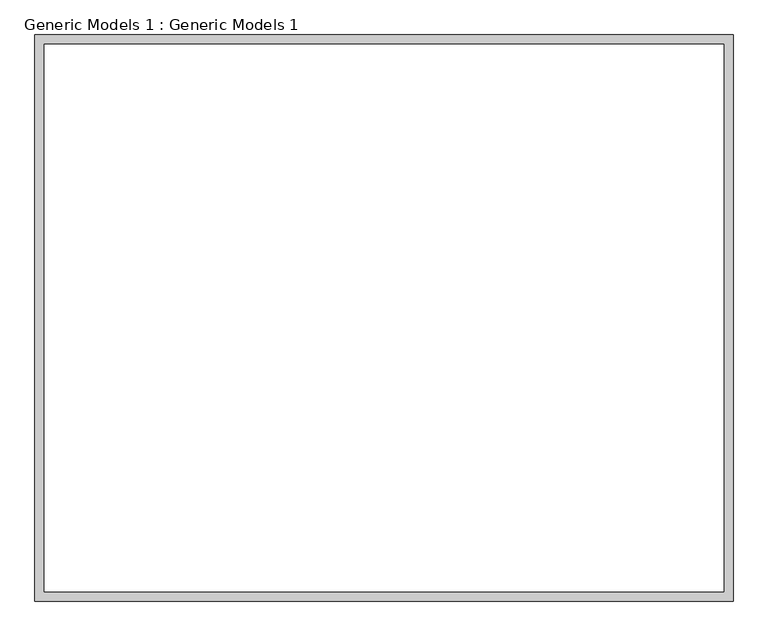
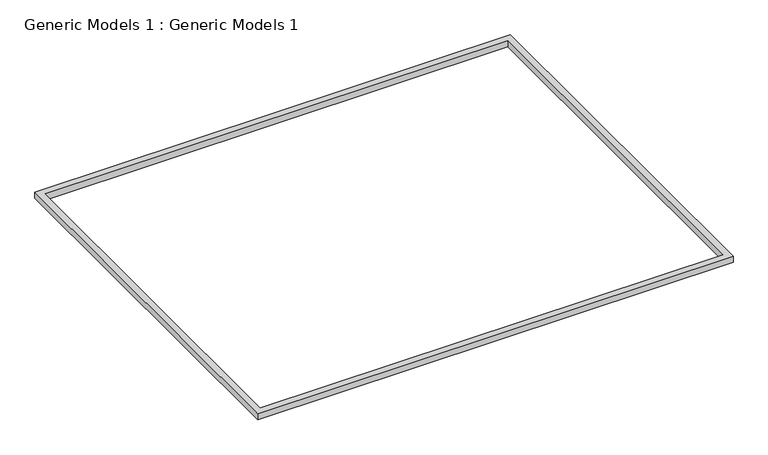
"""IFC4 building model written with IfcOpenShell, lengths in millimetres: proxy geometry, Generic Models 1 : Generic Models 1."""

from ifc_helpers import new_model, si_unit, frame, origin, place, context, project, spatial, polyline, outline, extrude, source, transform, mapped, element, save


def generic_models_1_generic_models_1_a1fc493f(model_context):
    return source(origin(), model_context, "Body", "SweptSolid", [
        extrude(outline(polyline([(-13365.3436606, 11380.4975873), (-13365.3436606, 8332.4975873), (-17124.5436606, 8332.4975873), (-17124.5436606, 11380.4975873), (-13365.3436606, 11380.4975873)]), holes=[polyline([(-13416.1436606, 11329.6975873), (-17073.7436606, 11329.6975873), (-17073.7436606, 8383.2975873), (-13416.1436606, 8383.2975873), (-13416.1436606, 11329.6975873)])]), frame((0.0, 0.0, 3048.0), z_axis=(0.0, 0.0, 1.0), x_axis=(1.0, 0.0, 0.0)), (0.0, 0.0, 1.0), 50.8),
    ])


if __name__ == "__main__":
    model = new_model("IFC4")
    model_context = context("Model", 3, world=origin())
    ifc_project = project(units=[si_unit("LENGTHUNIT", "METRE", prefix="MILLI")], contexts=[model_context])
    site = spatial("IfcSite", under=ifc_project)
    building = spatial("IfcBuilding", under=site)
    placement = place(None, origin())
    generic_models_1_generic_models_1_shape = generic_models_1_generic_models_1_a1fc493f(model_context)
    element("IfcBuildingElementProxy", 1, Name="Generic Models 1 : Generic Models 1", ObjectType="Generic Models 1 : Generic Models 1", at=placement, inside=building, context=model_context, shape_type="MappedRepresentation", body=[
        mapped(generic_models_1_generic_models_1_shape, transform((0.0, 0.0, 0.0), x_axis=(1.0, 0.0, 0.0), y_axis=(0.0, 1.0, 0.0), z_axis=(0.0, 0.0, 1.0))),
    ])
    save(model, "model.ifc")

# Revit data of these elements
# Element 1 (IfcBuildingElementProxy, "Generic Models 1 : Generic Models 1")
#   Materials on its faces: "Porcelain, Linen"
# Materials
#   "Porcelain, Linen": class "Ceramic", colour RGB 120 120 120, transparency 0, Description = "Porcelain, linen", Cost = 0
